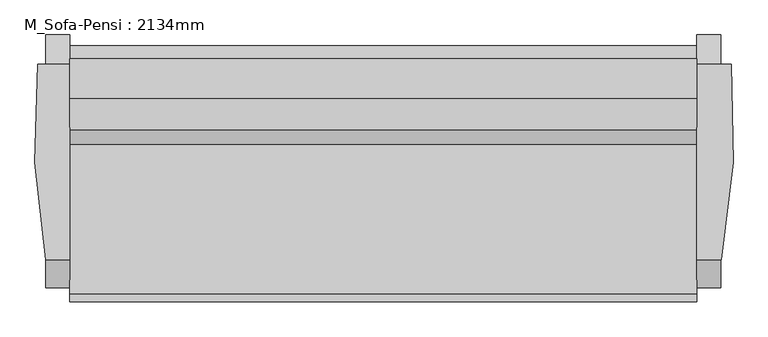
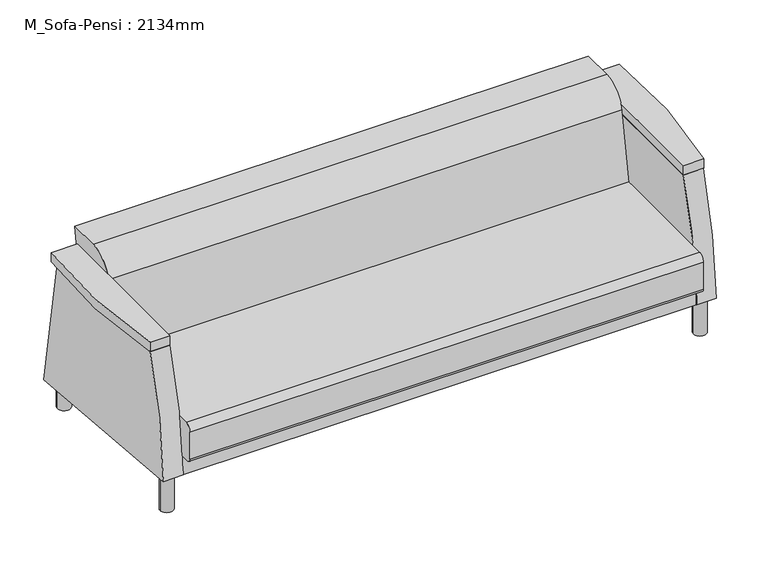
"""IFC4 building model written with IfcOpenShell, lengths in millimetres: furniture geometry, M_Sofa-Pensi : 2134mm."""

from ifc_helpers import new_model, si_unit, point, frame, frame_2d, origin, origin_with_axes, place, context, project, spatial, polyline, circle_curve, trimmed, segment, composite_curve, outline, extrude, source, transform, mapped, element, save
from ifc_brep_helpers import plane_surface, cylinder_surface, advanced_brep


def m_sofa_pensi_2134mm_538a523a(model_context):
    return source(origin(), model_context, "Body", "SolidModel", [
        extrude(outline(composite_curve([segment(trimmed(circle_curve(frame_2d((-116.5901639, 351.2509954)), 25.4), [point((-141.9901639, 351.2509954))], [point((-116.5901639, 376.6509954))], False, "CARTESIAN"), True, "CONTINUOUS"), segment(polyline([(-116.5901639, 376.6509954), (355.3895541, 376.6509954), (402.1988177, 642.1195211)]), True, "CONTINUOUS"), segment(trimmed(circle_curve(frame_2d((502.2552854, 624.4768662)), 101.6), [point((402.1988177, 642.1195211))], [point((502.2552854, 726.0768662))], False, "CARTESIAN"), True, "CONTINUOUS"), segment(polyline([(502.2552854, 726.0768662), (626.3344485, 726.0768662), (609.5377828, 620.1719187), (667.6541767, 224.2509954), (-126.1151639, 224.2509954)]), True, "CONTINUOUS"), segment(trimmed(circle_curve(frame_2d((-126.1151639, 240.1259954)), 15.875), [point((-126.1151639, 224.2509954))], [point((-141.9901639, 240.1259954))], False, "CARTESIAN"), True, "CONTINUOUS"), segment(polyline([(-141.9901639, 240.1259954), (-141.9901639, 351.2509954)]), True, "CONTINUOUS")], self_intersect=False)), frame((-712.19375, 0.0, 0.0), z_axis=(1.0, 0.0, 0.0), x_axis=(0.0, 1.0, 0.0)), (0.0, 0.0, 1.0), 1981.6),
        extrude(outline(composite_curve([segment(trimmed(circle_curve(frame_2d((-750.29375, -53.0901639)), 25.4), [point((-775.69375, -53.0901639))], [point((-724.89375, -53.0901639))], False, "CARTESIAN"), True, "CONTINUOUS"), segment(trimmed(circle_curve(frame_2d((-750.29375, -53.0901639)), 25.4), [point((-724.89375, -53.0901639))], [point((-775.69375, -53.0901639))], False, "CARTESIAN"), True, "CONTINUOUS")], self_intersect=False)), origin_with_axes(), (0.0, 0.0, 1.0), 148.43125),
        extrude(outline(composite_curve([segment(trimmed(circle_curve(frame_2d((-750.29375, 632.7098361)), 25.4), [point((-775.69375, 632.7098361))], [point((-724.89375, 632.7098361))], False, "CARTESIAN"), True, "CONTINUOUS"), segment(trimmed(circle_curve(frame_2d((-750.29375, 632.7098361)), 25.4), [point((-724.89375, 632.7098361))], [point((-775.69375, 632.7098361))], False, "CARTESIAN"), True, "CONTINUOUS")], self_intersect=False)), origin_with_axes(), (0.0, 0.0, 1.0), 148.43125),
        extrude(outline(composite_curve([segment(trimmed(circle_curve(frame_2d((1307.50625, 632.7098361)), 25.4), [point((1282.10625, 632.7098361))], [point((1332.90625, 632.7098361))], False, "CARTESIAN"), True, "CONTINUOUS"), segment(trimmed(circle_curve(frame_2d((1307.50625, 632.7098361)), 25.4), [point((1332.90625, 632.7098361))], [point((1282.10625, 632.7098361))], False, "CARTESIAN"), True, "CONTINUOUS")], self_intersect=False)), origin_with_axes(), (0.0, 0.0, 1.0), 148.43125),
        extrude(outline(composite_curve([segment(trimmed(circle_curve(frame_2d((1307.50625, -53.0901639)), 25.4), [point((1282.10625, -53.0901639))], [point((1332.90625, -53.0901639))], False, "CARTESIAN"), True, "CONTINUOUS"), segment(trimmed(circle_curve(frame_2d((1307.50625, -53.0901639)), 25.4), [point((1332.90625, -53.0901639))], [point((1282.10625, -53.0901639))], False, "CARTESIAN"), True, "CONTINUOUS")], self_intersect=False)), origin_with_axes(), (0.0, 0.0, 1.0), 148.43125),
        advanced_brep(
        [(1345.60625, 701.7619204, 79.3588346), (1345.60625, 608.6917937, 626.0203985), (1345.60625, -9.3943348, 626.0203985), (1345.60625, -97.7900405, 149.3105671), (1269.40625, -9.3943348, 626.0203985), (1269.40625, 608.6917937, 626.0203985), (1269.40625, 701.7619204, 79.3588346), (1269.40625, -83.3930704, 148.0509954), (1269.40625, 668.3047863, 148.0509954), (1269.40625, 668.3047863, 224.2509954), (1269.40625, -93.6952137, 224.2509954), (1269.40625, -93.6952137, 148.9523161), (1269.40625, -97.7900405, 149.3105671), (1269.40625, -93.6952137, 148.0509954), (-712.19375, -83.3930704, 148.0509954), (-712.19375, -93.6952137, 148.0509954), (-712.19375, -93.6952137, 148.9523161), (-712.19375, 668.3047863, 224.2509954), (-712.19375, -93.6952137, 224.2509954), (-712.19375, 668.3047863, 148.0509954), (-712.19375, 701.7619204, 79.3588346), (-712.19375, 608.6917937, 626.0203985), (-712.19375, -9.3943348, 626.0203985), (-712.19375, -97.7900405, 149.3105671), (-788.39375, -9.3943348, 626.0203985), (-788.39375, 608.6917937, 626.0203985), (-788.39375, 701.7619204, 79.3588346), (-788.39375, -97.7900405, 149.3105671)],
        [
            (0, 1),
            (1, 2),
            (2, 3, circle_curve(frame((1345.60625, 1499.9783711, 99.5888442), z_axis=(1.0, 0.0, 0.0), x_axis=(0.0, 1.0, 0.0)), 1598.5418814)),
            (3, 0),
            (4, 5),
            (5, 6),
            (6, 7),
            (7, 8),
            (8, 9),
            (9, 10),
            (10, 4, circle_curve(frame((1269.40625, 1499.9783711, 99.5888442), z_axis=(-1.0, 0.0, 0.0), x_axis=(0.0, 1.0, 0.0)), 1598.5418814)),
            (11, 12),
            (12, 10, circle_curve(frame((1269.40625, 1499.9783711, 99.5888442), z_axis=(-1.0, 0.0, 0.0), x_axis=(0.0, 1.0, 0.0)), 1598.5418814)),
            (10, 11),
            (0, 6),
            (5, 1),
            (4, 2),
            (12, 3),
            (11, 7),
            (11, 13),
            (13, 7),
            (14, 15),
            (15, 16),
            (16, 14),
            (9, 17),
            (17, 18),
            (18, 10),
            (18, 16),
            (15, 13),
            (14, 19),
            (19, 8),
            (19, 17),
            (20, 21),
            (21, 22),
            (22, 18, circle_curve(frame((-712.19375, 1499.9783711, 99.5888442), z_axis=(1.0, 0.0, 0.0), x_axis=(0.0, 1.0, 0.0)), 1598.5418814)),
            (14, 20),
            (18, 23, circle_curve(frame((-712.19375, 1499.9783711, 99.5888442), z_axis=(1.0, 0.0, 0.0), x_axis=(0.0, 1.0, 0.0)), 1598.5418814)),
            (23, 16),
            (24, 25),
            (25, 26),
            (26, 27),
            (27, 24, circle_curve(frame((-788.39375, 1499.9783711, 99.5888442), z_axis=(-1.0, 0.0, 0.0), x_axis=(0.0, 1.0, 0.0)), 1598.5418814)),
            (27, 23),
            (22, 24),
            (26, 20),
            (25, 21),
        ],
        [
            plane_surface(frame((1345.60625, 608.6917937, 626.0203985), z_axis=(1.0000000000000002, 0.0, 0.0), x_axis=(0.0, -0.16783676484789783, 0.985814800236531))),
            plane_surface(frame((1269.40625, 608.6917937, 626.0203985), z_axis=(-1.0000000000000002, 0.0, 0.0), x_axis=(0.0, 0.16783676484789783, -0.985814800236531))),
            plane_surface(frame((1345.60625, 701.7619204, 79.3588346), z_axis=(0.0, 0.985814800236531, 0.16783676484789783), x_axis=(-1.0, 0.0, 0.0))),
            plane_surface(frame((1345.60625, 608.6917937, 626.0203985), z_axis=(0.0, 0.0, 1.0), x_axis=(-1.0, 0.0, 0.0))),
            cylinder_surface(frame((1269.40625, 1499.9783711, 99.5888442), z_axis=(1.0, 0.0, 0.0), x_axis=(0.0, 1.0, 0.0)), 1598.5418814),
            plane_surface(frame((1345.60625, -97.7900405, 149.3105671), z_axis=(0.0, -0.08715574274767213, -0.9961946980917444), x_axis=(-1.0, 0.0, 0.0))),
            plane_surface(frame((1269.40625, -93.6952137, 224.2509954), z_axis=(1.0, 0.0, 0.0), x_axis=(0.0, -1.0, 0.0))),
            plane_surface(frame((-712.19375, -93.6952137, 224.2509954), z_axis=(-1.0, 0.0, 0.0), x_axis=(0.0, 1.0, 0.0))),
            plane_surface(frame((1269.40625, 668.3047863, 224.2509954), z_axis=(0.0, 0.0, 1.0), x_axis=(-1.0, 0.0, 0.0))),
            plane_surface(frame((1269.40625, -93.6952137, 224.2509954), z_axis=(0.0, -1.0, 0.0), x_axis=(-1.0, 0.0, 0.0))),
            plane_surface(frame((1269.40625, -93.6952137, 148.0509954), z_axis=(0.0, 0.0, -1.0), x_axis=(-1.0, 0.0, 0.0))),
            plane_surface(frame((1269.40625, 668.3047863, 148.0509954), z_axis=(0.0, 1.0, 0.0), x_axis=(-1.0, 0.0, 0.0))),
            plane_surface(frame((-712.19375, 3098.5202525, 99.5888442), z_axis=(1.0, 0.0, 0.0), x_axis=(0.0, 0.0, 1.0))),
            plane_surface(frame((-788.39375, 3098.5202525, 99.5888442), z_axis=(-1.0, 0.0, 0.0), x_axis=(0.0, 0.0, -1.0))),
            cylinder_surface(frame((-788.39375, 1499.9783711, 99.5888442), z_axis=(1.0, 0.0, 0.0), x_axis=(0.0, 1.0, 0.0)), 1598.5418814),
            plane_surface(frame((-712.19375, -97.7900405, 149.3105671), z_axis=(0.0, -0.08715574274766119, -0.9961946980917453), x_axis=(-1.0, 0.0, 0.0))),
            plane_surface(frame((-712.19375, 701.7619204, 79.3588346), z_axis=(0.0, 0.9858148002365317, 0.16783676484789375), x_axis=(-1.0, 0.0, 0.0))),
            plane_surface(frame((-712.19375, 608.6917937, 626.0203985), z_axis=(0.0, 0.0, 1.0), x_axis=(-1.0, 0.0, 0.0))),
        ],
        [
            (0, [[1, 2, 3, 4]]),
            (1, [[5, 6, 7, 8, 9, 10, 11]]),
            (1, [[12, 13, 14]]),
            (2, [[-1, 15, -6, 16]]),
            (3, [[-2, -16, -5, 17]]),
            (4, [[-3, -17, -11, -13, 18]]),
            (5, [[-4, -18, -12, 19, -7, -15]]),
            (6, [[20, 21, -19]]),
            (7, [[22, 23, 24]]),
            (8, [[25, 26, 27, -10]]),
            (9, [[-27, 28, -23, 29, -20, -14]]),
            (10, [[-29, -22, 30, 31, -8, -21]]),
            (11, [[-25, -9, -31, 32]]),
            (12, [[33, 34, 35, -26, -32, -30, 36]]),
            (12, [[37, 38, -28]]),
            (13, [[39, 40, 41, 42]]),
            (14, [[-42, 43, -37, -35, 44]]),
            (15, [[-41, 45, -36, -24, -38, -43]]),
            (16, [[-33, -45, -40, 46]]),
            (17, [[-34, -46, -39, -44]]),
        ],
    ),
        extrude(outline(composite_curve([segment(polyline([(-712.19375, -9.3943348), (-788.39375, -9.3943348)]), True, "CONTINUOUS"), segment(trimmed(circle_curve(frame_2d((1379.7527561, 389.2697363)), 2204.4936638), [point((-788.39375, -9.3943348))], [point((-813.79375, 608.6917935))], False, "CARTESIAN"), True, "CONTINUOUS"), segment(polyline([(-813.79375, 608.6917935), (-712.19375, 608.6917935), (-712.19375, -9.3943348)]), True, "CONTINUOUS")], self_intersect=False)), frame((0.0, 0.0, 626.0203985), z_axis=(0.0, 0.0, 1.0), x_axis=(1.0, 0.0, 0.0)), (0.0, 0.0, 1.0), 38.1),
        extrude(outline(composite_curve([segment(polyline([(1269.40625, -9.3943348), (1269.40625, 608.9395268), (1378.0864453, 608.9395268)]), True, "CONTINUOUS"), segment(trimmed(circle_curve(frame_2d((-821.5771494, 407.0270204)), 2208.9111775), [point((1378.0864453, 608.9395268))], [point((1347.7273117, -9.3943348))], False, "CARTESIAN"), True, "CONTINUOUS"), segment(polyline([(1347.7273117, -9.3943348), (1269.40625, -9.3943348)]), True, "CONTINUOUS")], self_intersect=False)), frame((0.0, 0.0, 626.0203985), z_axis=(0.0, 0.0, 1.0), x_axis=(1.0, 0.0, 0.0)), (0.0, 0.0, 1.0), 38.1),
    ])


if __name__ == "__main__":
    model = new_model("IFC4")
    model_context = context("Model", 3, world=origin())
    ifc_project = project(units=[si_unit("LENGTHUNIT", "METRE", prefix="MILLI")], contexts=[model_context])
    site = spatial("IfcSite", under=ifc_project)
    building = spatial("IfcBuilding", under=site)
    placement = place(None, origin())
    m_sofa_pensi_2134mm_shape = m_sofa_pensi_2134mm_538a523a(model_context)
    element("IfcFurniture", 1, ObjectType="M_Sofa-Pensi : 2134mm", at=placement, inside=building, context=model_context, shape_type="MappedRepresentation", body=[
        mapped(m_sofa_pensi_2134mm_shape, transform((0.0, 0.0, 0.0), x_axis=(1.0, 0.0, 0.0), y_axis=(0.0, 1.0, 0.0), z_axis=(0.0, 0.0, 1.0))),
    ])
    save(model, "model.ifc")

# Revit data of these elements
# Type "M_Sofa-Pensi : 2134mm"
#   Length = 7.001312 ft
#   Sofa Material = Linen, Beige
#   Frame Material = Steel, Chrome Plated
#   Default Elevation = 0
# Element 1 (IfcFurniture, "M_Sofa-Pensi : 2134mm")
#   Materials on its faces: "Linen, Beige", "Steel, Chrome Plated"
# Materials
#   "Linen, Beige": class "Textile", colour RGB 249 239 230, transparency 0, Description = "Linen, beige", Cost = 0
#   "Steel, Chrome Plated": class "Metal", colour RGB 17 17 17, transparency 0, Description = "Chromiuim plated steel", Cost = 0
